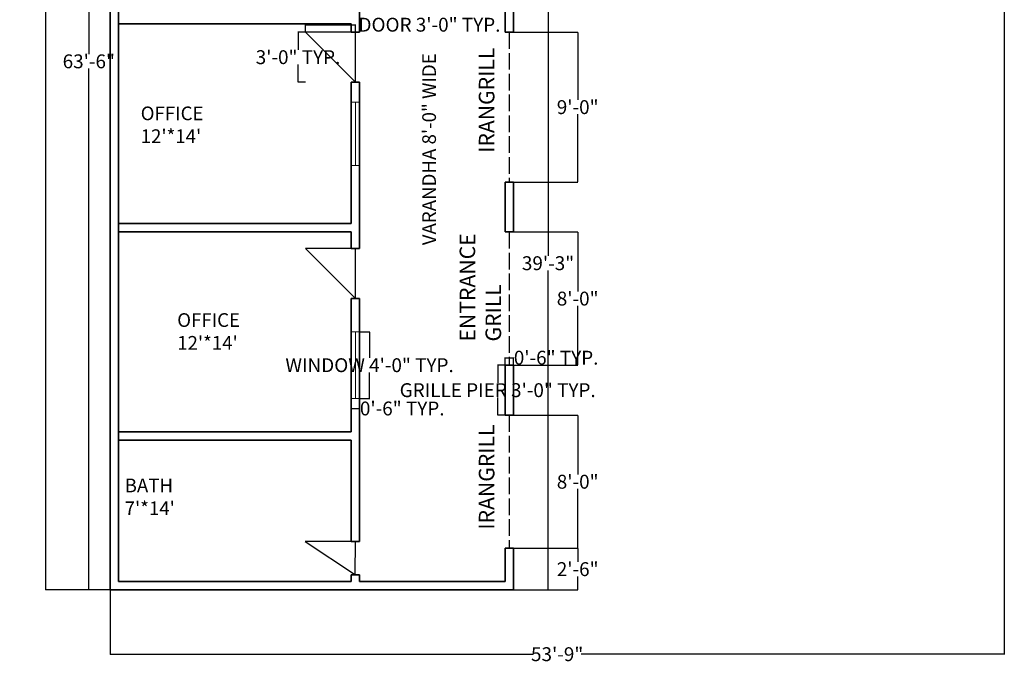
# Model space of a CAD drawing. Units: inches. Extents: x 20 to 815, y -31 to 943.
# Tile 1 of 2: x 20 to 730, y -31 to 433. Entities that reach past the tile are written whole.
import ezdxf

# ---------------------------------------------------------------- set-up
doc = ezdxf.new("R2010")
doc.units = ezdxf.units.IN
doc.header["$MEASUREMENT"] = 0
doc.linetypes.add('ACAD_ISO02W100', pattern=[15, 12, -3])
for name, color, linetype, lineweight in [('A-ANNO-DIMS', 2, 'Continuous', 18), ('A-ANNO-TEXT', 7, 'Continuous', 18), ('A-AREA-IDEN', 7, 'Continuous', 18), ('A-DOOR', 3, 'Continuous', 25), ('A-FLOR-GRIL', 8, 'ACAD_ISO02W100', 25), ('A-GLAZ', 4, 'Continuous', 18), ('A-WALL', 7, 'Continuous', 35)]:
    doc.layers.add(name, color=color, linetype=linetype, lineweight=lineweight)
doc.styles.get("Standard").update_dxf_attribs({"font": 'arial.ttf'})
doc.dimstyles.get("Standard").update_dxf_attribs({"dimtxt": 10, "dimasz": 0.18, "dimexe": 0.18, "dimexo": 0.0625, "dimgap": 0.09, "dimtad": 0, "dimtih": 1, "dimtoh": 1, "dimdec": 0, "dimzin": 0, "dimdsep": 46, "dimlunit": 3, "dimtxsty": 'Standard', "dimcen": 0.09, "dimadec": 0, "dimazin": 0, "dimtfac": 1, "dimtdec": 0, "dimtofl": 0, "dimtmove": 0, "dimatfit": 3, "dimfxl": 1, "dimtolj": 1, "dimtzin": 0, "dimarcsym": 0})

# ---------------------------------------------------------------- blocks, each defined once
blk = doc.blocks.new('*D6')
at = {"layer": 'A-ANNO-DIMS', "color": 0, "lineweight": -2, "transparency": 16777216}
for p, q in [((84.99, 783.99), (69.56, 783.99)), ((69.74, 783.81), (69.74, 408.19)), ((69.74, 22.17), (69.74, 397.79)), ((84.99, 21.99), (69.56, 21.99))]:
    blk.add_line(p, q, dxfattribs=at)
at = {"layer": 'A-ANNO-DIMS', "color": 0, "transparency": 16777216}
for points in [[(69.71, 783.81), (69.77, 783.81), (69.74, 783.99)], [(69.71, 22.17), (69.77, 22.17), (69.74, 21.99)]]:
    blk.add_solid(points, dxfattribs=at)
at = {"layer": 'Defpoints', "color": 0, "transparency": 16777216}
for p in [(69.74, 783.99), (85.05, 783.99), (85.05, 21.99)]:
    blk.add_point(p, dxfattribs=at)
at = {"layer": 'A-ANNO-DIMS', "color": 0, "transparency": 16777216, "insert": (69.74, 402.99), "char_height": 10, "attachment_point": 5}
blk.add_mtext('\\A1;63\'-6"', dxfattribs=at)
blk = doc.blocks.new('*D9')
at = {"layer": 'A-ANNO-DIMS', "color": 0, "lineweight": -2, "transparency": 16777216}
for p, q in [((376.11, 492.99), (401.14, 492.99)), ((400.96, 492.81), (400.96, 262.69)), ((400.96, 22.17), (400.96, 252.29)), ((376.11, 21.99), (401.14, 21.99))]:
    blk.add_line(p, q, dxfattribs=at)
at = {"layer": 'A-ANNO-DIMS', "color": 0, "transparency": 16777216}
for points in [[(400.93, 492.81), (400.99, 492.81), (400.96, 492.99)], [(400.93, 22.17), (400.99, 22.17), (400.96, 21.99)]]:
    blk.add_solid(points, dxfattribs=at)
at = {"layer": 'Defpoints', "color": 0, "transparency": 16777216}
for p in [(376.05, 492.99), (376.05, 21.99), (400.96, 21.99)]:
    blk.add_point(p, dxfattribs=at)
at = {"layer": 'A-ANNO-DIMS', "color": 0, "transparency": 16777216, "insert": (400.96, 257.49), "char_height": 10, "attachment_point": 5}
blk.add_mtext('\\A1;39\'-3"', dxfattribs=at)
blk = doc.blocks.new('DOOR-SINGLE-36')
for p, q in [((0, 0), (-36, 0)), ((-36, 0), (0, -36)), ((0, -36), (0, 0))]:
    blk.add_line(p, q)
blk = doc.blocks.new('WIN-48')
for p, q in [((-3, 48), (3, 48)), ((0, 0), (0, 48)), ((-3, 0), (3, 0))]:
    blk.add_line(p, q)
blk = doc.blocks.new('GRILLE-PIER-6X36')
for p, q in [((0, 36), (6, 36)), ((0, 36), (0, 0)), ((6, 36), (6, 0)), ((0, 0), (6, 0))]:
    blk.add_line(p, q)
blk = doc.blocks.new('*D16')
at = {"layer": 'A-ANNO-DIMS', "color": 0, "lineweight": -2, "transparency": 16777216}
for p, q in [((265.11, 207.99), (272.43, 207.99)), ((272.25, 207.81), (272.25, 189.26)), ((272.25, 160.17), (272.25, 178.73)), ((265.11, 159.99), (272.43, 159.99))]:
    blk.add_line(p, q, dxfattribs=at)
at = {"layer": 'A-ANNO-DIMS', "color": 0, "transparency": 16777216}
for points in [[(272.22, 207.81), (272.28, 207.81), (272.25, 207.99)], [(272.22, 160.17), (272.28, 160.17), (272.25, 159.99)]]:
    blk.add_solid(points, dxfattribs=at)
at = {"layer": 'Defpoints', "color": 0, "transparency": 16777216}
for p in [(265.05, 207.99), (272.25, 207.99), (265.05, 159.99)]:
    blk.add_point(p, dxfattribs=at)
at = {"layer": 'A-ANNO-DIMS', "color": 0, "transparency": 16777216, "insert": (272.25, 183.99), "char_height": 10, "attachment_point": 5}
blk.add_mtext('\\A1;WINDOW 4\'-0" TYP.', dxfattribs=at)
blk = doc.blocks.new('*D17')
at = {"layer": 'A-ANNO-DIMS', "color": 0, "lineweight": -2, "transparency": 16777216}
for p, q in [((259.05, 159.93), (259.05, 152.61)), ((265.05, 159.93), (265.05, 152.61)), ((259.23, 152.79), (264.87, 152.79)), ((265.05, 152.79), (265.23, 152.79))]:
    blk.add_line(p, q, dxfattribs=at)
at = {"layer": 'A-ANNO-DIMS', "color": 0, "transparency": 16777216}
for points in [[(259.23, 152.82), (259.23, 152.76), (259.05, 152.79)], [(264.87, 152.82), (264.87, 152.76), (265.05, 152.79)]]:
    blk.add_solid(points, dxfattribs=at)
at = {"layer": 'Defpoints', "color": 0, "transparency": 16777216}
for p in [(259.05, 159.99), (265.05, 159.99), (265.05, 152.79)]:
    blk.add_point(p, dxfattribs=at)
at = {"layer": 'A-ANNO-DIMS', "color": 0, "transparency": 16777216, "insert": (295.8, 152.79), "char_height": 10, "attachment_point": 5}
blk.add_mtext('\\A1;0\'-6" TYP.', dxfattribs=at)
blk = doc.blocks.new('*D24')
at = {"layer": 'A-ANNO-DIMS', "color": 0, "lineweight": -2, "transparency": 16777216}
for p, q in [((226.05, 424.05), (226.05, 429.57)), ((226.23, 429.39), (261.87, 429.39)), ((262.05, 424.05), (262.05, 429.57)), ((262.05, 429.39), (262.23, 429.39))]:
    blk.add_line(p, q, dxfattribs=at)
at = {"layer": 'A-ANNO-DIMS', "color": 0, "transparency": 16777216}
for points in [[(226.23, 429.42), (226.23, 429.36), (226.05, 429.39)], [(261.87, 429.42), (261.87, 429.36), (262.05, 429.39)]]:
    blk.add_solid(points, dxfattribs=at)
at = {"layer": 'Defpoints', "color": 0, "transparency": 16777216}
for p in [(262.05, 429.39), (226.05, 423.99), (262.05, 423.99)]:
    blk.add_point(p, dxfattribs=at)
at = {"layer": 'A-ANNO-DIMS', "color": 0, "transparency": 16777216, "insert": (315.45, 429.39), "char_height": 10, "attachment_point": 5}
blk.add_mtext('\\A1;DOOR 3\'-0" TYP.', dxfattribs=at)
blk = doc.blocks.new('*D25')
at = {"layer": 'A-ANNO-DIMS', "color": 0, "lineweight": -2, "transparency": 16777216}
for p, q in [((225.99, 423.99), (220.47, 423.99)), ((220.65, 423.81), (220.65, 411.19)), ((220.65, 388.17), (220.65, 400.79)), ((225.99, 387.99), (220.47, 387.99))]:
    blk.add_line(p, q, dxfattribs=at)
at = {"layer": 'A-ANNO-DIMS', "color": 0, "transparency": 16777216}
for points in [[(220.62, 423.81), (220.68, 423.81), (220.65, 423.99)], [(220.62, 388.17), (220.68, 388.17), (220.65, 387.99)]]:
    blk.add_solid(points, dxfattribs=at)
at = {"layer": 'Defpoints', "color": 0, "transparency": 16777216}
for p in [(220.65, 423.99), (226.05, 423.99), (226.05, 387.99)]:
    blk.add_point(p, dxfattribs=at)
at = {"layer": 'A-ANNO-DIMS', "color": 0, "transparency": 16777216, "insert": (220.65, 405.99), "char_height": 10, "attachment_point": 5}
blk.add_mtext('\\A1;3\'-0" TYP.', dxfattribs=at)
blk = doc.blocks.new('*D26')
at = {"layer": 'A-ANNO-DIMS', "color": 0, "lineweight": -2, "transparency": 16777216}
for p, q in [((369.99, 183.99), (364.47, 183.99)), ((364.65, 183.81), (364.65, 171.26)), ((364.65, 148.17), (364.65, 160.73)), ((369.99, 147.99), (364.47, 147.99))]:
    blk.add_line(p, q, dxfattribs=at)
at = {"layer": 'A-ANNO-DIMS', "color": 0, "transparency": 16777216}
for points in [[(364.62, 183.81), (364.68, 183.81), (364.65, 183.99)], [(364.62, 148.17), (364.68, 148.17), (364.65, 147.99)]]:
    blk.add_solid(points, dxfattribs=at)
at = {"layer": 'Defpoints', "color": 0, "transparency": 16777216}
for p in [(364.65, 183.99), (370.05, 183.99), (370.05, 147.99)]:
    blk.add_point(p, dxfattribs=at)
at = {"layer": 'A-ANNO-DIMS', "color": 0, "transparency": 16777216, "insert": (364.65, 165.99), "char_height": 10, "attachment_point": 5}
blk.add_mtext('\\A1;GRILLE PIER 3\'-0" TYP.', dxfattribs=at)
blk = doc.blocks.new('*D27')
at = {"layer": 'A-ANNO-DIMS', "color": 0, "lineweight": -2, "transparency": 16777216}
for p, q in [((370.05, 184.05), (370.05, 189.57)), ((370.23, 189.39), (375.87, 189.39)), ((376.05, 184.05), (376.05, 189.57)), ((376.05, 189.39), (376.23, 189.39))]:
    blk.add_line(p, q, dxfattribs=at)
at = {"layer": 'A-ANNO-DIMS', "color": 0, "transparency": 16777216}
for points in [[(370.23, 189.42), (370.23, 189.36), (370.05, 189.39)], [(375.87, 189.42), (375.87, 189.36), (376.05, 189.39)]]:
    blk.add_solid(points, dxfattribs=at)
at = {"layer": 'Defpoints', "color": 0, "transparency": 16777216}
for p in [(376.05, 189.39), (370.05, 183.99), (376.05, 183.99)]:
    blk.add_point(p, dxfattribs=at)
at = {"layer": 'A-ANNO-DIMS', "color": 0, "transparency": 16777216, "insert": (406.8, 189.39), "char_height": 10, "attachment_point": 5}
blk.add_mtext('\\A1;0\'-6" TYP.', dxfattribs=at)
blk = doc.blocks.new('*D28')
at = {"layer": 'A-ANNO-DIMS', "color": 0, "lineweight": -2, "transparency": 16777216}
for p, q in [((730.05, 492.93), (730.05, -24.49)), ((85.05, 21.93), (85.05, -24.49)), ((85.23, -24.31), (390.29, -24.31)), ((729.87, -24.31), (424.82, -24.31))]:
    blk.add_line(p, q, dxfattribs=at)
at = {"layer": 'A-ANNO-DIMS', "color": 0, "transparency": 16777216}
for points in [[(85.23, -24.28), (85.23, -24.34), (85.05, -24.31)], [(729.87, -24.28), (729.87, -24.34), (730.05, -24.31)]]:
    blk.add_solid(points, dxfattribs=at)
at = {"layer": 'Defpoints', "color": 0, "transparency": 16777216}
for p in [(730.05, 492.99), (85.05, 21.99), (730.05, -24.31)]:
    blk.add_point(p, dxfattribs=at)
at = {"layer": 'A-ANNO-DIMS', "color": 0, "transparency": 16777216, "insert": (407.55, -24.31), "char_height": 10, "attachment_point": 5}
blk.add_mtext('\\A1;53\'-9"', dxfattribs=at)
blk = doc.blocks.new('*D29')
at = {"layer": 'A-ANNO-DIMS', "color": 0, "lineweight": -2, "transparency": 16777216}
for p, q in [((180.99, 876.99), (38.57, 876.99)), ((38.75, 876.81), (38.75, 454.69)), ((38.75, 22.17), (38.75, 444.29)), ((84.99, 21.99), (38.57, 21.99))]:
    blk.add_line(p, q, dxfattribs=at)
at = {"layer": 'A-ANNO-DIMS', "color": 0, "transparency": 16777216}
for points in [[(38.72, 876.81), (38.78, 876.81), (38.75, 876.99)], [(38.72, 22.17), (38.78, 22.17), (38.75, 21.99)]]:
    blk.add_solid(points, dxfattribs=at)
at = {"layer": 'Defpoints', "color": 0, "transparency": 16777216}
for p in [(38.75, 876.99), (181.05, 876.99), (85.05, 21.99)]:
    blk.add_point(p, dxfattribs=at)
at = {"layer": 'A-ANNO-DIMS', "color": 0, "transparency": 16777216, "insert": (38.75, 449.49), "char_height": 10, "attachment_point": 5}
blk.add_mtext('\\A1;71\'-3"', dxfattribs=at)
blk = doc.blocks.new('*D30')
at = {"layer": 'A-ANNO-DIMS', "color": 0, "lineweight": -2, "transparency": 16777216}
for p, q in [((376.11, 51.99), (422.53, 51.99)), ((422.35, 51.81), (422.35, 42.19)), ((422.35, 22.17), (422.35, 31.8)), ((376.11, 21.99), (422.53, 21.99))]:
    blk.add_line(p, q, dxfattribs=at)
at = {"layer": 'A-ANNO-DIMS', "color": 0, "transparency": 16777216}
for points in [[(422.32, 51.81), (422.38, 51.81), (422.35, 51.99)], [(422.32, 22.17), (422.38, 22.17), (422.35, 21.99)]]:
    blk.add_solid(points, dxfattribs=at)
at = {"layer": 'Defpoints', "color": 0, "transparency": 16777216}
for p in [(376.05, 51.99), (376.05, 21.99), (422.35, 21.99)]:
    blk.add_point(p, dxfattribs=at)
at = {"layer": 'A-ANNO-DIMS', "color": 0, "transparency": 16777216, "insert": (422.35, 36.99), "char_height": 10, "attachment_point": 5}
blk.add_mtext('\\A1;2\'-6"', dxfattribs=at)
blk = doc.blocks.new('*D31')
at = {"layer": 'A-ANNO-DIMS', "color": 0, "lineweight": -2, "transparency": 16777216}
for p, q in [((376.11, 147.99), (422.53, 147.99)), ((422.35, 147.81), (422.35, 105.19)), ((422.35, 52.17), (422.35, 94.8)), ((376.11, 51.99), (422.53, 51.99))]:
    blk.add_line(p, q, dxfattribs=at)
at = {"layer": 'A-ANNO-DIMS', "color": 0, "transparency": 16777216}
for points in [[(422.32, 147.81), (422.38, 147.81), (422.35, 147.99)], [(422.32, 52.17), (422.38, 52.17), (422.35, 51.99)]]:
    blk.add_solid(points, dxfattribs=at)
at = {"layer": 'Defpoints', "color": 0, "transparency": 16777216}
for p in [(376.05, 147.99), (376.05, 51.99), (422.35, 51.99)]:
    blk.add_point(p, dxfattribs=at)
at = {"layer": 'A-ANNO-DIMS', "color": 0, "transparency": 16777216, "insert": (422.35, 99.99), "char_height": 10, "attachment_point": 5}
blk.add_mtext('\\A1;8\'-0"', dxfattribs=at)
blk = doc.blocks.new('*D32')
at = {"layer": 'A-ANNO-DIMS', "color": 0, "lineweight": -2, "transparency": 16777216}
for p, q in [((376.11, 279.99), (422.53, 279.99)), ((422.35, 279.81), (422.35, 237.19)), ((422.35, 184.17), (422.35, 226.8)), ((376.11, 183.99), (422.53, 183.99))]:
    blk.add_line(p, q, dxfattribs=at)
at = {"layer": 'A-ANNO-DIMS', "color": 0, "transparency": 16777216}
for points in [[(422.32, 279.81), (422.38, 279.81), (422.35, 279.99)], [(422.32, 184.17), (422.38, 184.17), (422.35, 183.99)]]:
    blk.add_solid(points, dxfattribs=at)
at = {"layer": 'Defpoints', "color": 0, "transparency": 16777216}
for p in [(376.05, 279.99), (376.05, 183.99), (422.35, 183.99)]:
    blk.add_point(p, dxfattribs=at)
at = {"layer": 'A-ANNO-DIMS', "color": 0, "transparency": 16777216, "insert": (422.35, 231.99), "char_height": 10, "attachment_point": 5}
blk.add_mtext('\\A1;8\'-0"', dxfattribs=at)
blk = doc.blocks.new('*D33')
at = {"layer": 'A-ANNO-DIMS', "color": 0, "lineweight": -2, "transparency": 16777216}
for p, q in [((376.11, 423.99), (422.53, 423.99)), ((422.35, 423.81), (422.35, 375.19)), ((422.35, 316.17), (422.35, 364.8)), ((376.11, 315.99), (422.53, 315.99))]:
    blk.add_line(p, q, dxfattribs=at)
at = {"layer": 'A-ANNO-DIMS', "color": 0, "transparency": 16777216}
for points in [[(422.32, 423.81), (422.38, 423.81), (422.35, 423.99)], [(422.32, 316.17), (422.38, 316.17), (422.35, 315.99)]]:
    blk.add_solid(points, dxfattribs=at)
at = {"layer": 'Defpoints', "color": 0, "transparency": 16777216}
for p in [(376.05, 423.99), (376.05, 315.99), (422.35, 315.99)]:
    blk.add_point(p, dxfattribs=at)
at = {"layer": 'A-ANNO-DIMS', "color": 0, "transparency": 16777216, "insert": (422.35, 369.99), "char_height": 10, "attachment_point": 5}
blk.add_mtext('\\A1;9\'-0"', dxfattribs=at)

msp = doc.modelspace()

# ---------------------------------------------------------------- linework, layer by layer
at = {"layer": 'A-DOOR'}
for p, q in [((262.05, 56.99), (225.77, 56.99)), ((225.77, 56.99), (262.05, 32.99)), ((261.83, 33.59), (262.05, 56.99))]:
    msp.add_line(p, q, dxfattribs=at)
at = {"layer": 'A-FLOR-GRIL'}
for p, q in [((373.05, 423.99), (373.05, 315.99)), ((373.05, 279.99), (373.05, 183.99)), ((373.05, 147.99), (373.05, 51.99))]:
    msp.add_line(p, q, dxfattribs=at)
at = {"layer": 'A-GLAZ'}
for p, q in [((265.05, 373.65), (259.05, 373.65)), ((262.05, 327.99), (262.05, 373.65)), ((265.05, 327.99), (265.05, 373.65)), ((259.05, 327.99), (265.05, 327.99))]:
    msp.add_line(p, q, dxfattribs=at)
at = {"layer": 'A-WALL'}
for p, q in [((85.05, 21.99), (85.05, 783.99)), ((91.05, 27.99), (91.05, 777.99)), ((265.05, 423.99), (265.05, 567.99)), ((370.05, 498.99), (370.05, 423.99)), ((376.05, 492.99), (376.05, 423.99)), ((91.05, 429.99), (259.05, 429.99)), ((259.05, 423.99), (259.05, 429.99)), ((259.05, 423.99), (265.05, 423.99)), ((370.05, 423.99), (376.05, 423.99)), ((259.05, 387.99), (265.05, 387.99)), ((259.05, 285.99), (259.05, 387.99)), ((265.05, 267.99), (265.05, 387.99)), ((376.05, 315.99), (376.05, 279.99)), ((91.05, 285.99), (259.05, 285.99)), ((91.05, 279.99), (259.05, 279.99)), ((259.05, 267.99), (259.05, 279.99)), ((259.05, 267.99), (265.05, 267.99)), ((259.05, 231.99), (265.05, 231.99)), ((259.05, 135.99), (259.05, 231.99)), ((265.05, 56.99), (265.05, 231.99)), ((91.05, 135.99), (259.05, 135.99)), ((91.05, 129.99), (259.05, 129.99)), ((259.05, 56.99), (259.05, 129.99)), ((265.05, 56.99), (259.05, 56.99)), ((370.05, 27.99), (370.05, 51.99)), ((370.05, 51.99), (376.05, 51.99)), ((370.05, 51.99), (370.05, 27.99)), ((376.05, 51.99), (376.05, 21.99)), ((259.05, 27.99), (259.05, 32.99)), ((265.05, 32.99), (259.05, 32.99)), ((265.05, 27.99), (265.05, 32.99)), ((376.05, 21.99), (85.05, 21.99)), ((259.05, 27.99), (91.05, 27.99)), ((370.05, 27.99), (265.05, 27.99))]:
    msp.add_line(p, q, dxfattribs=at)

# ---------------------------------------------------------------- block references
at = {"layer": 'A-DOOR'}
for p in [(262.05, 423.99), (262.05, 267.99)]:
    msp.add_blockref('DOOR-SINGLE-36', p, dxfattribs=at)
at = {"layer": 'A-GLAZ'}
msp.add_blockref('WIN-48', (262.05, 159.99), dxfattribs=at)
at = {"layer": 'A-WALL', "rotation": 180}
msp.add_blockref('GRILLE-PIER-6X36', (376.05, 315.99), dxfattribs=at)
at = {"layer": 'A-WALL'}
msp.add_blockref('GRILLE-PIER-6X36', (370.05, 147.99), dxfattribs=at)

# ---------------------------------------------------------------- texts
at = {"layer": 'A-ANNO-TEXT', "attachment_point": 1, "rotation": 90}
for s, insert, char_height in [('IRANGRILL', (351.05, 337.08), 11.194), ('ENTRANCE GRILL', (337.22, 201.06), 11.1945), ('IRANGRILL', (351.05, 65.47), 11.194)]:
    msp.add_mtext_dynamic_manual_height_columns(s, width=35.9978, gutter_width=55.97, heights=[0], dxfattribs=dict(at, insert=insert, char_height=char_height))
at = {"layer": 'A-AREA-IDEN', "insert": (310.25, 270.44), "char_height": 9.8677, "attachment_point": 1, "rotation": 90}
msp.add_mtext('VARANDHA 8\'-0" WIDE', dxfattribs=at)
at = {"layer": 'A-AREA-IDEN', "char_height": 9.868, "attachment_point": 1}
for s, insert in [("OFFICE\\P12'*14'", (107.17, 370.42)), ("OFFICE\\P12'*14'", (133.5, 221.46)), ("BATH\\P7'*14'", (95.61, 102.24))]:
    msp.add_mtext(s, dxfattribs=dict(at, insert=insert))

# ---------------------------------------------------------------- dimensions: what is measured, and where the dimension line sits
at = {"layer": 'A-ANNO-DIMS'}
for base, p1, p2, angle, override, picture, middle in [((38.75, 876.99), (85.05, 21.99), (181.05, 876.99), 90, {"dimdec": 1, "dimlfac": 1, "dimrnd": 0, "dimzin": 1, "dimdsep": 46, "dimlunit": 4, "dimfrac": 2}, '*D29', (38.75, 449.49)), ((69.74, 783.99), (85.05, 21.99), (85.05, 783.99), 90, {"dimclrd": 0, "dimclre": 0, "dimclrt": 0}, '*D6', (69.74, 402.99)), ((400.96, 21.99), (376.05, 492.99), (376.05, 21.99), 90, {"dimclrd": 0, "dimclre": 0, "dimclrt": 0}, '*D9', (400.96, 257.49)), ((422.35, 315.99), (376.05, 423.99), (376.05, 315.99), 270, {"dimdec": 1, "dimlfac": 1, "dimrnd": 0, "dimzin": 1, "dimdsep": 46, "dimlunit": 4, "dimfrac": 2}, '*D33', (422.35, 369.99)), ((422.35, 183.99), (376.05, 279.99), (376.05, 183.99), 270, {"dimdec": 1, "dimlfac": 1, "dimrnd": 0, "dimzin": 1, "dimdsep": 46, "dimlunit": 4, "dimfrac": 2}, '*D32', (422.35, 231.99)), ((422.35, 51.99), (376.05, 147.99), (376.05, 51.99), 270, {"dimdec": 1, "dimlfac": 1, "dimrnd": 0, "dimzin": 1, "dimdsep": 46, "dimlunit": 4, "dimfrac": 2}, '*D31', (422.35, 99.99)), ((422.35, 21.99), (376.05, 51.99), (376.05, 21.99), 270, {"dimdec": 1, "dimlfac": 1, "dimrnd": 0, "dimzin": 1, "dimdsep": 46, "dimlunit": 4, "dimfrac": 2}, '*D30', (422.35, 36.99))]:
    dim = msp.add_linear_dim(base=base, p1=p1, p2=p2, angle=angle, dimstyle='Standard', override=override, dxfattribs=at)
    dim.commit()
    dim.dimension.update_dxf_attribs({"geometry": picture, "text_midpoint": middle})
dim = msp.add_linear_dim(base=(730.05, -24.31), p1=(85.05, 21.99), p2=(730.05, 492.99), dimstyle='Standard', override={"dimdec": 1, "dimlfac": 1, "dimrnd": 0, "dimzin": 1, "dimdsep": 46, "dimlunit": 4, "dimfrac": 2}, dxfattribs=at)
dim.commit()
dim.dimension.update_dxf_attribs({"geometry": '*D28', "text_midpoint": (407.55, -24.31)})
for base, p1, p2, text, picture, middle in [((262.05, 429.39), (226.05, 423.99), (262.05, 423.99), 'DOOR <> TYP.', '*D24', (315.45, 429.39)), ((376.05, 189.39), (370.05, 183.99), (376.05, 183.99), '<> TYP.', '*D27', (406.8, 189.39)), ((265.05, 152.79), (259.05, 159.99), (265.05, 159.99), '<> TYP.', '*D17', (295.8, 152.79))]:
    dim = msp.add_linear_dim(base=base, p1=p1, p2=p2, text=text, dimstyle='Standard', override={"dimdec": 1, "dimlfac": 1, "dimrnd": 0, "dimzin": 1, "dimdsep": 46, "dimlunit": 4, "dimfrac": 2}, dxfattribs=at)
    dim.commit()
    dim.dimension.update_dxf_attribs({"geometry": picture, "text_midpoint": middle})
for base, p1, p2, text, picture, middle in [((220.65, 423.99), (226.05, 387.99), (226.05, 423.99), '<> TYP.', '*D25', (220.65, 405.99)), ((272.25, 207.99), (265.05, 159.99), (265.05, 207.99), 'WINDOW <> TYP.', '*D16', (272.25, 183.99)), ((364.65, 183.99), (370.05, 147.99), (370.05, 183.99), 'GRILLE PIER <> TYP.', '*D26', (364.65, 165.99))]:
    dim = msp.add_linear_dim(base=base, p1=p1, p2=p2, angle=90, text=text, dimstyle='Standard', override={"dimdec": 1, "dimlfac": 1, "dimrnd": 0, "dimzin": 1, "dimdsep": 46, "dimlunit": 4, "dimfrac": 2}, dxfattribs=at)
    dim.commit()
    dim.dimension.update_dxf_attribs({"geometry": picture, "text_midpoint": middle})

doc.saveas('drawing.dxf')
